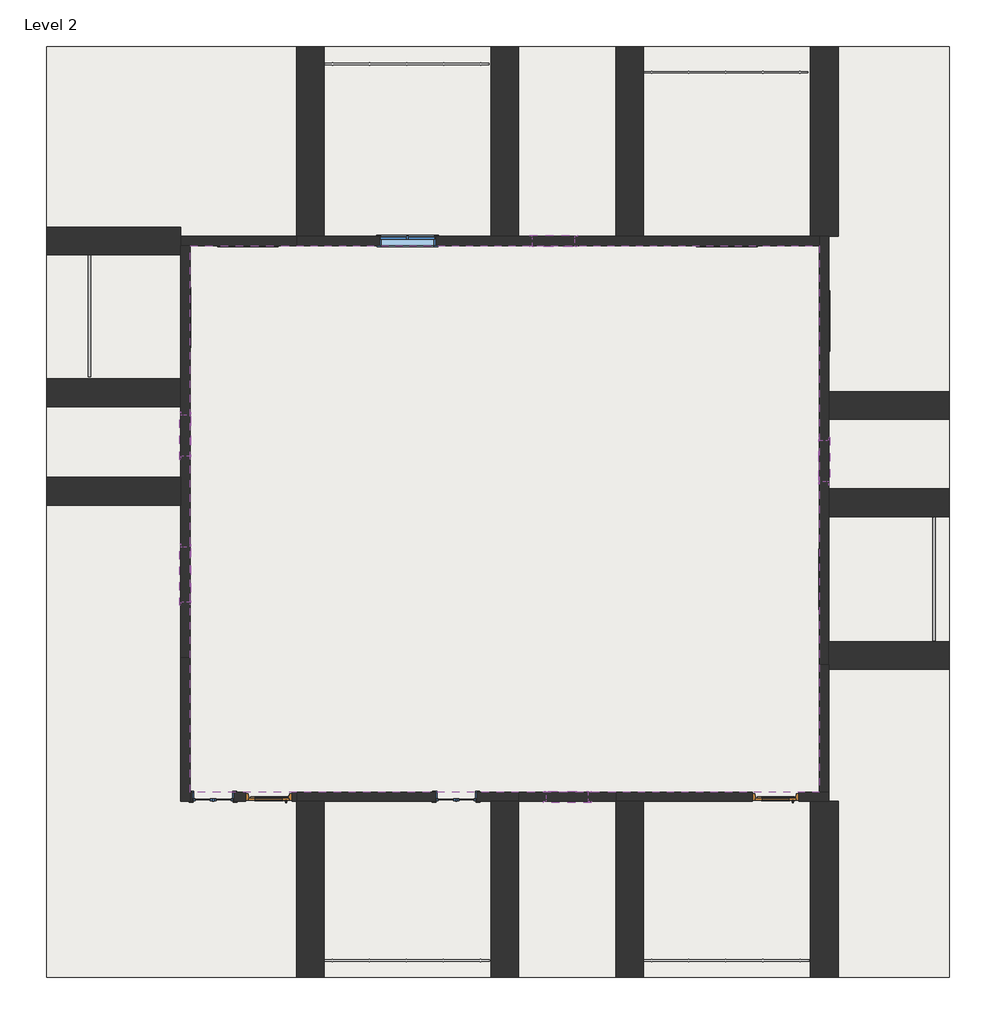
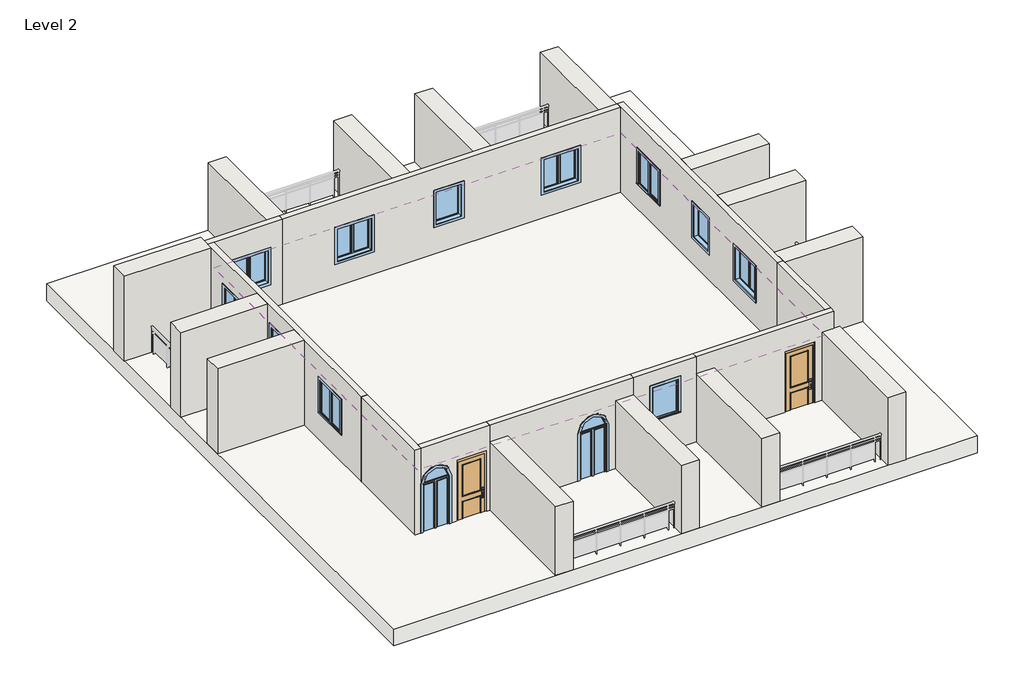
# One storey, part 1 of 2: 24 walls, 13 windows, 2 doors, 1 covering, 1 slab.
"""IFC4 building model written with IfcOpenShell, lengths in millimetres."""

from ifc_helpers import new_model, si_unit, point, frame, frame_2d, origin, place, context, project, spatial, polyline, circle_curve, trimmed, segment, composite_curve, outline, extrude, faceted_brep, transform, mapped, element, save
from ifc_brep_helpers import plane_surface, revolved_surface, advanced_brep
from components import door_b6c2ee01, window_4e95f2a8, window_0862ab64, window_3a1167bf, window_8a4441b2

model = new_model("IFC4")

# Units and contexts
model_context = context("Model", 3, world=origin())
ifc_project = project(units=[si_unit("LENGTHUNIT", "METRE", prefix="MILLI")], contexts=[model_context])

# Site, building, storey
site = spatial("IfcSite", under=ifc_project)
building = spatial("IfcBuilding", under=site)
storey = spatial("IfcBuildingStorey", under=building, Name="Level 2", Elevation=3048.0)

# Covering
placement = place(None, origin())
element("IfcCovering", 1, ObjectType="2' x 4' ACT System", at=placement, inside=storey, context=model_context, shape_type="SweptSolid", body=[
    extrude(outline(polyline([(-12179.4937431, 6319.013611), (-9842.6937431, 6319.013611), (1638.1062569, 6319.013611), (1638.1062569, -2875.786389), (1638.1062569, -5669.786389), (-2832.2937431, -5669.786389), (-4965.8937431, -5669.786389), (-9842.6937431, -5669.786389), (-12179.4937431, -5669.786389), (-12179.4937431, -2723.386389), (-12179.4937431, 6319.013611)])), frame((0.0, 0.0, 5486.4), z_axis=(0.0, 0.0, 1.0), x_axis=(1.0, 0.0, 0.0)), (0.0, 0.0, 1.0), 57.15),
])

# Doors
door_shape = door_b6c2ee01(model_context)
element("IfcDoor", 2, ObjectType="Door-Exterior-Single-Two_Lite : 36\" x 94\"", at=placement, inside=storey, context=model_context, shape_type="MappedRepresentation", body=[
    mapped(door_shape, transform((-10452.2937431, -5765.036389, 3048.0), x_axis=(-1.0, 0.0, 0.0), y_axis=(0.0, -1.0, 0.0), z_axis=(0.0, 0.0, 1.0))),
])
element("IfcDoor", 3, ObjectType="Door-Exterior-Single-Two_Lite : 36\" x 94\"", at=placement, inside=storey, context=model_context, shape_type="MappedRepresentation", body=[
    mapped(door_shape, transform((672.9062569, -5765.036389, 3048.0), x_axis=(-1.0, 0.0, 0.0), y_axis=(0.0, -1.0, 0.0), z_axis=(0.0, 0.0, 1.0))),
])

# Slab
element("IfcSlab", 4, ObjectType="Generic - 2' 4", at=placement, inside=storey, context=model_context, shape_type="SweptSolid", body=[
    extrude(outline(polyline([(4482.9062569, 10687.813611), (4482.9062569, -9733.786389), (-15329.0937431, -9733.786389), (-15329.0937431, 10687.813611), (4482.9062569, 10687.813611)])), frame((0.0, 0.0, 2743.2), z_axis=(0.0, 0.0, 1.0), x_axis=(1.0, 0.0, 0.0)), (0.0, 0.0, 1.0), 609.6),
])

# Walls
element("IfcWall", 5, ObjectType="Generic - 8\"", at=placement, inside=storey, context=model_context, shape_type="Brep", body=[
    faceted_brep([(-12382.6937431, 6319.013611, 3352.8), (-12179.4937431, 6319.013611, 3352.8), (-9842.6937431, 6319.013611, 3352.8), (-9842.6937431, 6319.013611, 6400.8), (-12179.4937431, 6319.013611, 6400.8), (-12382.6937431, 6319.013611, 6400.8), (-10299.8937431, 6319.013611, 5486.4), (-10299.8937431, 6319.013611, 4267.2), (-11519.0937431, 6319.013611, 4267.2), (-11519.0937431, 6319.013611, 5486.4), (-12382.6937431, 6522.213611, 3352.8), (-12382.6937431, 6522.213611, 6400.8), (-9842.6937431, 6522.213611, 6400.8), (-9842.6937431, 6522.213611, 3352.8), (-10299.8937431, 6522.213611, 5486.4), (-11519.0937431, 6522.213611, 5486.4), (-11519.0937431, 6522.213611, 4267.2), (-10299.8937431, 6522.213611, 4267.2)], [[[0, 1, 2, 3, 4, 5], [6, 7, 8, 9]], [[10, 11, 12, 13], [14, 15, 16, 17]], [[2, 1, 0, 10, 13]], [[3, 2, 13, 12]], [[5, 4, 3, 12, 11]], [[0, 5, 11, 10]], [[7, 6, 14, 17]], [[8, 7, 17, 16]], [[9, 8, 16, 15]], [[6, 9, 15, 14]]]),
])
element("IfcWall", 6, ObjectType="Generic - 8\"", at=placement, inside=storey, context=model_context, shape_type="Brep", body=[
    faceted_brep([(-12179.4937431, -5872.986389, 3352.8), (-12179.4937431, -5669.786389, 3352.8), (-12179.4937431, -2723.386389, 3352.8), (-12179.4937431, -2723.386389, 6400.8), (-12179.4937431, -5669.786389, 6400.8), (-12179.4937431, -5872.986389, 6400.8), (-12382.6937431, -5872.986389, 3352.8), (-12382.6937431, -5872.986389, 6400.8), (-12382.6937431, -2723.386389, 6400.8), (-12382.6937431, -2723.386389, 3352.8)], [[[0, 1, 2, 3, 4, 5]], [[6, 7, 8, 9]], [[2, 1, 0, 6, 9]], [[3, 2, 9, 8]], [[5, 4, 3, 8, 7]], [[0, 5, 7, 6]]]),
])
element("IfcWall", 7, ObjectType="Generic - 8\"", at=placement, inside=storey, context=model_context, shape_type="Brep", body=[
    faceted_brep([(-2832.2937431, -5669.786389, 3352.8), (-2832.2937431, -5669.786389, 6400.8), (1638.1062569, -5669.786389, 6400.8), (1841.3062569, -5669.786389, 6400.8), (1841.3062569, -5669.786389, 3352.8), (1638.1062569, -5669.786389, 3352.8), (1180.9062569, -5669.786389, 3352.8), (1180.9062569, -5669.786389, 5537.2), (164.9062569, -5669.786389, 5537.2), (164.9062569, -5669.786389, 3352.8), (-2832.2937431, -5872.986389, 6400.8), (-2832.2937431, -5872.986389, 5798.8571637), (-2832.2937431, -5872.986389, 3352.8), (-2222.6937431, -5872.986389, 3352.8), (164.9062569, -5872.986389, 3352.8), (164.9062569, -5872.986389, 5537.2), (1180.9062569, -5872.986389, 5537.2), (1180.9062569, -5872.986389, 3352.8), (1434.9062569, -5872.986389, 3352.8), (1841.3062569, -5872.986389, 3352.8), (1841.3062569, -5872.986389, 6400.8)], [[[0, 1, 2, 3, 4, 5, 6, 7, 8, 9]], [[10, 11, 12, 13, 14, 15, 16, 17, 18, 19, 20]], [[4, 19, 18, 17, 6, 5]], [[12, 0, 9, 14, 13]], [[1, 0, 12, 11, 10]], [[3, 2, 1, 10, 20]], [[3, 20, 19, 4]], [[8, 15, 14, 9]], [[15, 8, 7, 16]], [[16, 7, 6, 17]]]),
])
element("IfcWall", 8, ObjectType="Generic - 8\"", at=placement, inside=storey, context=model_context, shape_type="Brep", body=[
    faceted_brep([(1638.1062569, 6522.213611, 6400.8), (1638.1062569, 6522.213611, 3352.8), (1638.1062569, 6319.013611, 3352.8), (1638.1062569, -2875.786389, 3352.8), (1638.1062569, -2875.786389, 6400.8), (1638.1062569, 6319.013611, 6400.8), (1638.1062569, 1137.413611, 5557.6747769), (1638.1062569, 1137.413611, 4338.4747769), (1638.1062569, 2051.813611, 4338.4747769), (1638.1062569, 2051.813611, 5557.6747769), (1638.1062569, -1605.786389, 5497.5712595), (1638.1062569, -1605.786389, 4278.3712595), (1638.1062569, -386.586389, 4278.3712595), (1638.1062569, -386.586389, 5497.5712595), (1638.1062569, 4058.413611, 5497.5712595), (1638.1062569, 4058.413611, 4278.3712595), (1638.1062569, 5277.613611, 4278.3712595), (1638.1062569, 5277.613611, 5497.5712595), (1841.3062569, 6522.213611, 3352.8), (1841.3062569, 6522.213611, 6400.8), (1841.3062569, 3118.613611, 6400.8), (1841.3062569, 2509.013611, 6400.8), (1841.3062569, 985.013611, 6400.8), (1841.3062569, 375.413611, 6400.8), (1841.3062569, -2367.786389, 6400.8), (1841.3062569, -2875.786389, 6400.8), (1841.3062569, -2875.786389, 3352.8), (1841.3062569, -2367.786389, 3352.8), (1841.3062569, 375.413611, 3352.8), (1841.3062569, 985.013611, 3352.8), (1841.3062569, 2509.013611, 3352.8), (1841.3062569, 3118.613611, 3352.8), (1841.3062569, 1137.413611, 5557.6747769), (1841.3062569, 2051.813611, 5557.6747769), (1841.3062569, 2051.813611, 4338.4747769), (1841.3062569, 1137.413611, 4338.4747769), (1841.3062569, -1605.786389, 5497.5712595), (1841.3062569, -386.586389, 5497.5712595), (1841.3062569, -386.586389, 4278.3712595), (1841.3062569, -1605.786389, 4278.3712595), (1841.3062569, 4058.413611, 5497.5712595), (1841.3062569, 5277.613611, 5497.5712595), (1841.3062569, 5277.613611, 4278.3712595), (1841.3062569, 4058.413611, 4278.3712595)], [[[0, 1, 2, 3, 4, 5], [6, 7, 8, 9], [10, 11, 12, 13], [14, 15, 16, 17]], [[18, 19, 20, 21, 22, 23, 24, 25, 26, 27, 28, 29, 30, 31], [32, 33, 34, 35], [36, 37, 38, 39], [40, 41, 42, 43]], [[3, 2, 1, 18, 31, 30, 29, 28, 27, 26]], [[4, 3, 26, 25]], [[0, 5, 4, 25, 24, 23, 22, 21, 20, 19]], [[0, 19, 18, 1]], [[7, 6, 32, 35]], [[8, 7, 35, 34]], [[9, 8, 34, 33]], [[6, 9, 33, 32]], [[11, 10, 36, 39]], [[12, 11, 39, 38]], [[13, 12, 38, 37]], [[10, 13, 37, 36]], [[15, 14, 40, 43]], [[16, 15, 43, 42]], [[17, 16, 42, 41]], [[14, 17, 41, 40]]]),
])
element("IfcWall", 9, ObjectType="Generic - 8\"", at=placement, inside=storey, context=model_context, shape_type="Brep", body=[
    faceted_brep([(-12179.4937431, -2723.386389, 3352.8), (-12179.4937431, 6319.013611, 3352.8), (-12179.4937431, 6319.013611, 6400.8), (-12179.4937431, -2723.386389, 6400.8), (-12179.4937431, 2610.613611, 5723.7149116), (-12179.4937431, 2610.613611, 4504.5149116), (-12179.4937431, 1696.213611, 4504.5149116), (-12179.4937431, 1696.213611, 5723.7149116), (-12179.4937431, -284.986389, 5546.8059909), (-12179.4937431, -284.986389, 4327.6059909), (-12179.4937431, -1504.186389, 4327.6059909), (-12179.4937431, -1504.186389, 5546.8059909), (-12179.4937431, 5353.813611, 5473.1335827), (-12179.4937431, 5353.813611, 4253.9335827), (-12179.4937431, 4134.613611, 4253.9335827), (-12179.4937431, 4134.613611, 5473.1335827), (-12382.6937431, -2723.386389, 3352.8), (-12382.6937431, -2723.386389, 6400.8), (-12382.6937431, 629.413611, 6400.8), (-12382.6937431, 1239.013611, 6400.8), (-12382.6937431, 2788.413611, 6400.8), (-12382.6937431, 3398.013611, 6400.8), (-12382.6937431, 6115.813611, 6400.8), (-12382.6937431, 6319.013611, 6400.8), (-12382.6937431, 6319.013611, 3352.8), (-12382.6937431, 6115.813611, 3352.8), (-12382.6937431, 3398.013611, 3352.8), (-12382.6937431, 2788.413611, 3352.8), (-12382.6937431, 1239.013611, 3352.8), (-12382.6937431, 629.413611, 3352.8), (-12382.6937431, 2610.613611, 5723.7149116), (-12382.6937431, 1696.213611, 5723.7149116), (-12382.6937431, 1696.213611, 4504.5149116), (-12382.6937431, 2610.613611, 4504.5149116), (-12382.6937431, -284.986389, 5546.8059909), (-12382.6937431, -1504.186389, 5546.8059909), (-12382.6937431, -1504.186389, 4327.6059909), (-12382.6937431, -284.986389, 4327.6059909), (-12382.6937431, 5353.813611, 5473.1335827), (-12382.6937431, 4134.613611, 5473.1335827), (-12382.6937431, 4134.613611, 4253.9335827), (-12382.6937431, 5353.813611, 4253.9335827)], [[[0, 1, 2, 3], [4, 5, 6, 7], [8, 9, 10, 11], [12, 13, 14, 15]], [[16, 17, 18, 19, 20, 21, 22, 23, 24, 25, 26, 27, 28, 29], [30, 31, 32, 33], [34, 35, 36, 37], [38, 39, 40, 41]], [[1, 0, 16, 29, 28, 27, 26, 25, 24]], [[3, 2, 23, 22, 21, 20, 19, 18, 17]], [[0, 3, 17, 16]], [[2, 1, 24, 23]], [[5, 4, 30, 33]], [[6, 5, 33, 32]], [[7, 6, 32, 31]], [[4, 7, 31, 30]], [[9, 8, 34, 37]], [[10, 9, 37, 36]], [[11, 10, 36, 35]], [[8, 11, 35, 34]], [[13, 12, 38, 41]], [[14, 13, 41, 40]], [[15, 14, 40, 39]], [[12, 15, 39, 38]]]),
])
element("IfcWall", 10, ObjectType="Generic - 8\"", at=placement, inside=storey, context=model_context, shape_type="SweptSolid", body=[
    extrude(outline(composite_curve([segment(polyline([(6400.8, -9842.6937431), (6400.8, -12179.4937431), (3352.8, -12179.4937431), (3352.8, -12128.6937431), (5091.597687, -12128.6937431)]), True, "CONTINUOUS"), segment(trimmed(circle_curve(frame_2d((5091.597687, -11671.4937431)), 457.2), [point((5091.597687, -12128.6937431))], [point((5091.597687, -11214.2937431))], True, "CARTESIAN"), True, "CONTINUOUS"), segment(polyline([(5091.597687, -11214.2937431), (3352.8, -11214.2937431), (3352.8, -10960.2937431), (5537.2, -10960.2937431), (5537.2, -9944.2937431), (3352.8, -9944.2937431), (3352.8, -9842.6937431), (6400.8, -9842.6937431)]), True, "CONTINUOUS")], self_intersect=False)), frame((0.0, -5872.986389, 0.0), z_axis=(0.0, 1.0, 0.0), x_axis=(0.0, 0.0, 1.0)), (0.0, 0.0, 1.0), 203.2),
])
element("IfcWall", 11, ObjectType="Generic - 8\"", at=placement, inside=storey, context=model_context, shape_type="SweptSolid", body=[
    extrude(outline(polyline([(1638.1062569, -5669.786389), (1638.1062569, -2875.786389), (1841.3062569, -2875.786389), (1841.3062569, -5669.786389), (1638.1062569, -5669.786389)])), frame((0.0, 0.0, 3352.8), z_axis=(0.0, 0.0, 1.0), x_axis=(1.0, 0.0, 0.0)), (0.0, 0.0, 1.0), 3048.0),
])
element("IfcWall", 12, ObjectType="Generic - 8\"", at=placement, inside=storey, context=model_context, shape_type="Brep", body=[
    faceted_brep([(-9842.6937431, 6319.013611, 3352.8), (1638.1062569, 6319.013611, 3352.8), (1638.1062569, 6319.013611, 6400.8), (-9842.6937431, 6319.013611, 6400.8), (-3746.6937431, 6319.013611, 5584.3983257), (-3746.6937431, 6319.013611, 4365.1983257), (-4661.0937431, 6319.013611, 4365.1983257), (-4661.0937431, 6319.013611, 5584.3983257), (-6794.6937431, 6319.013611, 5433.182989), (-6794.6937431, 6319.013611, 4213.982989), (-8013.8937431, 6319.013611, 4213.982989), (-8013.8937431, 6319.013611, 5433.182989), (215.7062569, 6319.013611, 5470.4159819), (215.7062569, 6319.013611, 4251.2159819), (-1003.4937431, 6319.013611, 4251.2159819), (-1003.4937431, 6319.013611, 5470.4159819), (-9842.6937431, 6522.213611, 3352.8), (-9842.6937431, 6522.213611, 5791.2), (-9842.6937431, 6522.213611, 6400.8), (1638.1062569, 6522.213611, 6400.8), (1638.1062569, 6522.213611, 3352.8), (1434.9062569, 6522.213611, 3352.8), (-2222.6937431, 6522.213611, 3352.8), (-2832.2937431, 6522.213611, 3352.8), (-4965.8937431, 6522.213611, 3352.8), (-5575.4937431, 6522.213611, 3352.8), (-9233.0937431, 6522.213611, 3352.8), (-3746.6937431, 6522.213611, 5584.3983257), (-4661.0937431, 6522.213611, 5584.3983257), (-4661.0937431, 6522.213611, 4365.1983257), (-3746.6937431, 6522.213611, 4365.1983257), (-6794.6937431, 6522.213611, 5433.182989), (-8013.8937431, 6522.213611, 5433.182989), (-8013.8937431, 6522.213611, 4213.982989), (-6794.6937431, 6522.213611, 4213.982989), (215.7062569, 6522.213611, 5470.4159819), (-1003.4937431, 6522.213611, 5470.4159819), (-1003.4937431, 6522.213611, 4251.2159819), (215.7062569, 6522.213611, 4251.2159819)], [[[0, 1, 2, 3], [4, 5, 6, 7], [8, 9, 10, 11], [12, 13, 14, 15]], [[16, 17, 18, 19, 20, 21, 22, 23, 24, 25, 26], [27, 28, 29, 30], [31, 32, 33, 34], [35, 36, 37, 38]], [[1, 0, 16, 26, 25, 24, 23, 22, 21, 20]], [[3, 2, 19, 18]], [[0, 3, 18, 17, 16]], [[1, 20, 19, 2]], [[5, 4, 27, 30]], [[6, 5, 30, 29]], [[7, 6, 29, 28]], [[4, 7, 28, 27]], [[9, 8, 31, 34]], [[10, 9, 34, 33]], [[11, 10, 33, 32]], [[8, 11, 32, 31]], [[13, 12, 35, 38]], [[14, 13, 38, 37]], [[15, 14, 37, 36]], [[12, 15, 36, 35]]]),
])
element("IfcWall", 13, ObjectType="Generic - 8\"", at=placement, inside=storey, context=model_context, shape_type="SweptSolid", body=[
    extrude(outline(polyline([(3352.8, -2832.2937431), (6400.8, -2832.2937431), (6400.8, -4965.8937431), (3352.8, -4965.8937431), (3352.8, -2832.2937431)]), holes=[polyline([(5847.074951, -4356.2937431), (5847.074951, -3441.8937431), (4627.874951, -3441.8937431), (4627.874951, -4356.2937431), (5847.074951, -4356.2937431)])]), frame((0.0, -5872.986389, 0.0), z_axis=(0.0, 1.0, 0.0), x_axis=(0.0, 0.0, 1.0)), (0.0, 0.0, 1.0), 203.2),
])
element("IfcWall", 14, ObjectType="Generic - 8\"", at=placement, inside=storey, context=model_context, shape_type="AdvancedBrep", body=[
    advanced_brep(
    [(-9842.6937431, -5669.786389, 3352.8), (-9842.6937431, -5669.786389, 6400.8), (-4965.8937431, -5669.786389, 6400.8), (-4965.8937431, -5669.786389, 3352.8), (-5880.2937431, -5669.786389, 3352.8), (-5880.2937431, -5669.786389, 5048.25), (-6794.6937431, -5669.786389, 5048.25), (-6794.6937431, -5669.786389, 3352.8), (-9842.6937431, -5872.986389, 6400.8), (-9842.6937431, -5872.986389, 5811.7612992), (-9842.6937431, -5872.986389, 3352.8), (-9233.0937431, -5872.986389, 3352.8), (-6794.6937431, -5872.986389, 3352.8), (-6794.6937431, -5872.986389, 5048.25), (-5880.2937431, -5872.986389, 5048.25), (-5880.2937431, -5872.986389, 3352.8), (-5575.4937431, -5872.986389, 3352.8), (-4965.8937431, -5872.986389, 3352.8), (-4965.8937431, -5872.986389, 5791.2), (-4965.8937431, -5872.986389, 6400.8)],
    [
        (0, 1),
        (1, 2),
        (2, 3),
        (3, 4),
        (4, 5),
        (5, 6, circle_curve(frame((-6337.4937431, -5669.786389, 5048.25), z_axis=(0.0, -1.0, 0.0), x_axis=(-1.0, 0.0, 0.0)), 457.2)),
        (6, 7),
        (7, 0),
        (8, 9),
        (9, 10),
        (10, 11),
        (11, 12),
        (12, 13),
        (13, 14, circle_curve(frame((-6337.4937431, -5872.986389, 5048.25), z_axis=(0.0, 1.0, 0.0), x_axis=(-1.0, 0.0, 0.0)), 457.2)),
        (14, 15),
        (15, 16),
        (16, 17),
        (17, 18),
        (18, 19),
        (19, 8),
        (3, 17),
        (15, 4),
        (10, 0),
        (7, 12),
        (8, 1),
        (19, 2),
        (6, 13),
        (14, 5),
    ],
    [
        plane_surface(frame((1423.3958892, -5669.786389, 3352.8), z_axis=(0.0, 1.0, 0.0), x_axis=(-1.0, 0.0, 0.0))),
        plane_surface(frame((1423.3958892, -5872.986389, 3352.8), z_axis=(0.0, -1.0, 0.0), x_axis=(1.0, 0.0, 0.0))),
        plane_surface(frame((-4965.8937431, -5669.786389, 3352.8), z_axis=(0.0, 0.0, -1.0), x_axis=(0.0, -1.0, 0.0))),
        plane_surface(frame((-9842.6937431, -5669.786389, 3352.8), z_axis=(-1.0, 0.0, 0.0), x_axis=(0.0, -1.0, 0.0))),
        plane_surface(frame((-9842.6937431, -5669.786389, 6400.8), z_axis=(0.0, 0.0, 1.0), x_axis=(0.0, -1.0, 0.0))),
        plane_surface(frame((-4965.8937431, -5669.786389, 6400.8), z_axis=(1.0, 0.0, 0.0), x_axis=(0.0, -1.0, 0.0))),
        plane_surface(frame((-6794.6937431, -7193.786389, 5048.25), z_axis=(1.0, 0.0, 0.0), x_axis=(0.0, 1.0, 0.0))),
        plane_surface(frame((-5880.2937431, -7193.786389, 3200.4), z_axis=(-1.0, 0.0, 0.0), x_axis=(0.0, 1.0, 0.0))),
        revolved_surface(polyline([(-6794.6937431, -5872.986389, 5048.25), (-6794.6937431, -5669.786389, 5048.25)]), (-6337.4937431, -4145.786389, 5048.25), (0.0, -1.0, 0.0)),
    ],
    [
        (0, [[1, 2, 3, 4, 5, 6, 7, 8]]),
        (1, [[9, 10, 11, 12, 13, 14, 15, 16, 17, 18, 19, 20]]),
        (2, [[21, -17, -16, 22, -4]]),
        (2, [[23, -8, 24, -12, -11]]),
        (3, [[-1, -23, -10, -9, 25]]),
        (4, [[-2, -25, -20, 26]]),
        (5, [[-3, -26, -19, -18, -21]]),
        (6, [[27, -13, -24, -7]]),
        (7, [[28, -5, -22, -15]]),
        (8, [[-27, -6, -28, -14]]),
    ],
),
])
element("IfcWall", 15, ObjectType="Generic -2' 2", at=placement, inside=storey, context=model_context, shape_type="Brep", body=[
    faceted_brep([(-12382.6937431, 6725.413611, 3352.8), (-15329.0937431, 6725.413611, 3352.8), (-15329.0937431, 6725.413611, 6400.8), (-12382.6937431, 6725.413611, 6400.8), (-12382.6937431, 6115.813611, 3352.8), (-12382.6937431, 6115.813611, 6400.8), (-15329.0937431, 6115.813611, 6400.8), (-15329.0937431, 6115.813611, 3352.8), (-12382.6937431, 6522.213611, 3352.8), (-12382.6937431, 6319.013611, 3352.8), (-12382.6937431, 6319.013611, 6400.8), (-12382.6937431, 6522.213611, 6400.8)], [[[0, 1, 2, 3]], [[4, 5, 6, 7]], [[1, 0, 8, 9, 4, 7]], [[2, 1, 7, 6]], [[3, 2, 6, 5, 10, 11]], [[0, 3, 11, 10, 5, 4, 9, 8]]]),
])
element("IfcWall", 16, ObjectType="Generic -2' 2", at=placement, inside=storey, context=model_context, shape_type="SweptSolid", body=[
    extrude(outline(polyline([(-15329.0937431, 3398.013611), (-12382.6937431, 3398.013611), (-12382.6937431, 2788.413611), (-15329.0937431, 2788.413611), (-15329.0937431, 3398.013611)])), frame((0.0, 0.0, 3352.8), z_axis=(0.0, 0.0, 1.0), x_axis=(1.0, 0.0, 0.0)), (0.0, 0.0, 1.0), 3048.0),
])
element("IfcWall", 17, ObjectType="Generic -2' 2", at=placement, inside=storey, context=model_context, shape_type="SweptSolid", body=[
    extrude(outline(polyline([(-15329.0937431, 1239.013611), (-12382.6937431, 1239.013611), (-12382.6937431, 629.413611), (-15329.0937431, 629.413611), (-15329.0937431, 1239.013611)])), frame((0.0, 0.0, 3352.8), z_axis=(0.0, 0.0, 1.0), x_axis=(1.0, 0.0, 0.0)), (0.0, 0.0, 1.0), 3048.0),
])
element("IfcWall", 18, ObjectType="Generic -2' 2", at=placement, inside=storey, context=model_context, shape_type="Brep", body=[
    faceted_brep([(1841.3062569, -2977.386389, 3352.8), (4482.9062569, -2977.386389, 3352.8), (4482.9062569, -2977.386389, 6400.8), (1841.3062569, -2977.386389, 6400.8), (1841.3062569, -2367.786389, 3352.8), (1841.3062569, -2367.786389, 6400.8), (4482.9062569, -2367.786389, 6400.8), (4482.9062569, -2367.786389, 3352.8), (1841.3062569, -2875.786389, 3352.8), (1841.3062569, -2875.786389, 6400.8)], [[[0, 1, 2, 3]], [[4, 5, 6, 7]], [[1, 0, 8, 4, 7]], [[2, 1, 7, 6]], [[3, 2, 6, 5, 9]], [[0, 3, 9, 5, 4, 8]]]),
])
element("IfcWall", 19, ObjectType="Generic -2' 2", at=placement, inside=storey, context=model_context, shape_type="SweptSolid", body=[
    extrude(outline(polyline([(4482.9062569, 375.413611), (1841.3062569, 375.413611), (1841.3062569, 985.013611), (4482.9062569, 985.013611), (4482.9062569, 375.413611)])), frame((0.0, 0.0, 3352.8), z_axis=(0.0, 0.0, 1.0), x_axis=(1.0, 0.0, 0.0)), (0.0, 0.0, 1.0), 3048.0),
])
element("IfcWall", 20, ObjectType="Generic -2' 2", at=placement, inside=storey, context=model_context, shape_type="SweptSolid", body=[
    extrude(outline(polyline([(4482.9062569, 2509.013611), (1841.3062569, 2509.013611), (1841.3062569, 3118.613611), (4482.9062569, 3118.613611), (4482.9062569, 2509.013611)])), frame((0.0, 0.0, 3352.8), z_axis=(0.0, 0.0, 1.0), x_axis=(1.0, 0.0, 0.0)), (0.0, 0.0, 1.0), 3048.0),
])
element("IfcWall", 21, ObjectType="Generic -2' 3 red", at=placement, inside=storey, context=model_context, shape_type="Brep", body=[
    faceted_brep([(1434.9062569, -5872.986389, 3352.8), (1434.9062569, -9733.786389, 3352.8), (1434.9062569, -9733.786389, 5791.2), (1434.9062569, -5872.986389, 5791.2), (2044.5062569, -5872.986389, 3352.8), (2044.5062569, -5872.986389, 5791.2), (2044.5062569, -9733.786389, 5791.2), (2044.5062569, -9733.786389, 3352.8), (1841.3062569, -5872.986389, 3352.8)], [[[0, 1, 2, 3]], [[4, 5, 6, 7]], [[1, 0, 8, 4, 7]], [[2, 1, 7, 6]], [[3, 2, 6, 5]], [[0, 3, 5, 4, 8]]]),
])
element("IfcWall", 22, ObjectType="Generic -2' 3 red", at=placement, inside=storey, context=model_context, shape_type="SweptSolid", body=[
    extrude(outline(polyline([(-2832.2937431, -9733.786389), (-2832.2937431, -5872.986389), (-2222.6937431, -5872.986389), (-2222.6937431, -9733.786389), (-2832.2937431, -9733.786389)])), frame((0.0, 0.0, 3352.8), z_axis=(0.0, 0.0, 1.0), x_axis=(1.0, 0.0, 0.0)), (0.0, 0.0, 1.0), 2446.0571637),
])
element("IfcWall", 23, ObjectType="Generic -2' 3 red", at=placement, inside=storey, context=model_context, shape_type="SweptSolid", body=[
    extrude(outline(polyline([(-5575.4937431, -9733.786389), (-5575.4937431, -5872.986389), (-4965.8937431, -5872.986389), (-4965.8937431, -9733.786389), (-5575.4937431, -9733.786389)])), frame((0.0, 0.0, 3352.8), z_axis=(0.0, 0.0, 1.0), x_axis=(1.0, 0.0, 0.0)), (0.0, 0.0, 1.0), 2438.4),
])
element("IfcWall", 24, ObjectType="Generic -2' 3 red", at=placement, inside=storey, context=model_context, shape_type="SweptSolid", body=[
    extrude(outline(polyline([(-9842.6937431, -9733.786389), (-9842.6937431, -5872.986389), (-9233.0937431, -5872.986389), (-9233.0937431, -9733.786389), (-9842.6937431, -9733.786389)])), frame((0.0, 0.0, 3352.8), z_axis=(0.0, 0.0, 1.0), x_axis=(1.0, 0.0, 0.0)), (0.0, 0.0, 1.0), 2458.9612992),
])
element("IfcWall", 25, ObjectType="Generic -2' 3 red", at=placement, inside=storey, context=model_context, shape_type="SweptSolid", body=[
    extrude(outline(polyline([(-9233.0937431, 10687.813611), (-9233.0937431, 6522.213611), (-9842.6937431, 6522.213611), (-9842.6937431, 10687.813611), (-9233.0937431, 10687.813611)])), frame((0.0, 0.0, 3352.8), z_axis=(0.0, 0.0, 1.0), x_axis=(1.0, 0.0, 0.0)), (0.0, 0.0, 1.0), 2438.4),
])
element("IfcWall", 26, ObjectType="Generic -2' 3 red", at=placement, inside=storey, context=model_context, shape_type="SweptSolid", body=[
    extrude(outline(polyline([(-4965.8937431, 10687.813611), (-4965.8937431, 6522.213611), (-5575.4937431, 6522.213611), (-5575.4937431, 10687.813611), (-4965.8937431, 10687.813611)])), frame((0.0, 0.0, 3352.8), z_axis=(0.0, 0.0, 1.0), x_axis=(1.0, 0.0, 0.0)), (0.0, 0.0, 1.0), 2443.0998934),
])
element("IfcWall", 27, ObjectType="Generic -2' 3 red", at=placement, inside=storey, context=model_context, shape_type="SweptSolid", body=[
    extrude(outline(polyline([(-2222.6937431, 10687.813611), (-2222.6937431, 6522.213611), (-2832.2937431, 6522.213611), (-2832.2937431, 10687.813611), (-2222.6937431, 10687.813611)])), frame((0.0, 0.0, 3352.8), z_axis=(0.0, 0.0, 1.0), x_axis=(1.0, 0.0, 0.0)), (0.0, 0.0, 1.0), 2443.7584708),
])
element("IfcWall", 28, ObjectType="Generic -2' 3 red", at=placement, inside=storey, context=model_context, shape_type="Brep", body=[
    faceted_brep([(2044.5062569, 6522.213611, 3352.8), (2044.5062569, 10687.813611, 3352.8), (2044.5062569, 10687.813611, 5791.2), (2044.5062569, 6522.213611, 5791.2), (1434.9062569, 6522.213611, 3352.8), (1434.9062569, 6522.213611, 5791.2), (1434.9062569, 10687.813611, 5791.2), (1434.9062569, 10687.813611, 3352.8), (1841.3062569, 6522.213611, 3352.8), (1638.1062569, 6522.213611, 3352.8)], [[[0, 1, 2, 3]], [[4, 5, 6, 7]], [[1, 0, 8, 9, 4, 7]], [[2, 1, 7, 6]], [[3, 2, 6, 5]], [[0, 3, 5, 4, 9, 8]]]),
])

# Windows
window_shape = window_4e95f2a8(model_context)
element("IfcWindow", 29, ObjectType="36\" x 72\"", at=placement, inside=storey, context=model_context, shape_type="MappedRepresentation", body=[
    mapped(window_shape, transform((-11663.491585, -5771.386389, 2938.947687), x_axis=(-1.0, 0.0, 0.0), y_axis=(0.0, -1.0, 0.0), z_axis=(0.0, 0.0, 1.0))),
])
element("IfcWindow", 30, ObjectType="36\" x 72\"", at=placement, inside=storey, context=model_context, shape_type="MappedRepresentation", body=[
    mapped(window_shape, transform((-6329.491585, -5771.386389, 2895.6), x_axis=(-1.0, 0.0, 0.0), y_axis=(0.0, -1.0, 0.0), z_axis=(0.0, 0.0, 1.0))),
])
window_2_shape = window_0862ab64(model_context)
element("IfcWindow", 31, ObjectType="Casement Dbl with Trim.0001 : 48\" x 48\"", at=placement, inside=storey, context=model_context, shape_type="MappedRepresentation", body=[
    mapped(window_2_shape, transform((-12262.0437431, -894.586389, 3413.2059909), x_axis=(0.0, 1.0, 0.0), y_axis=(-1.0, 0.0, 0.0), z_axis=(0.0, 0.0, 1.0))),
])
element("IfcWindow", 32, ObjectType="Casement Dbl with Trim.0001 : 48\" x 48\"", at=placement, inside=storey, context=model_context, shape_type="MappedRepresentation", body=[
    mapped(window_2_shape, transform((-12262.0437431, 4744.213611, 3339.5335827), x_axis=(0.0, 1.0, 0.0), y_axis=(-1.0, 0.0, 0.0), z_axis=(0.0, 0.0, 1.0))),
])
element("IfcWindow", 33, ObjectType="Casement Dbl with Trim.0001 : 48\" x 48\"", at=placement, inside=storey, context=model_context, shape_type="MappedRepresentation", body=[
    mapped(window_2_shape, transform((-7404.2937431, 6401.563611, 3299.582989), x_axis=(1.0, 0.0, 0.0), y_axis=(0.0, 1.0, 0.0), z_axis=(0.0, 0.0, 1.0))),
])
element("IfcWindow", 34, ObjectType="Casement Dbl with Trim.0001 : 48\" x 48\"", at=placement, inside=storey, context=model_context, shape_type="MappedRepresentation", body=[
    mapped(window_2_shape, transform((-393.8937431, 6401.563611, 3336.8159819), x_axis=(1.0, 0.0, 0.0), y_axis=(0.0, 1.0, 0.0), z_axis=(0.0, 0.0, 1.0))),
])
element("IfcWindow", 35, ObjectType="Casement Dbl with Trim.0001 : 48\" x 48\"", at=placement, inside=storey, context=model_context, shape_type="MappedRepresentation", body=[
    mapped(window_2_shape, transform((1720.6562569, -996.186389, 3363.9712595), x_axis=(0.0, -1.0, 0.0), y_axis=(1.0, 0.0, 0.0), z_axis=(0.0, 0.0, 1.0))),
])
element("IfcWindow", 36, ObjectType="Casement Dbl with Trim.0001 : 48\" x 48\"", at=placement, inside=storey, context=model_context, shape_type="MappedRepresentation", body=[
    mapped(window_2_shape, transform((-10909.4937431, 6401.563611, 3352.8), x_axis=(1.0, 0.0, 0.0), y_axis=(0.0, 1.0, 0.0), z_axis=(0.0, 0.0, 1.0))),
])
window_3_shape = window_3a1167bf(model_context)
element("IfcWindow", 37, ObjectType="Casement Dbl with Trim.0001 : 48\" x 48\"", at=placement, inside=storey, context=model_context, shape_type="MappedRepresentation", body=[
    mapped(window_3_shape, transform((1758.7562569, 4668.013611, 3363.9712595), x_axis=(0.0, -1.0, 0.0), y_axis=(1.0, 0.0, 0.0), z_axis=(0.0, 0.0, 1.0))),
])
window_4_shape = window_8a4441b2(model_context)
element("IfcWindow", 38, ObjectType="Casement with Trim : 36\" x 48\"", at=placement, inside=storey, context=model_context, shape_type="MappedRepresentation", body=[
    mapped(window_4_shape, transform((-3899.0937431, -5771.386389, 3713.474951), x_axis=(-1.0, 0.0, 0.0), y_axis=(0.0, -1.0, 0.0), z_axis=(0.0, 0.0, 1.0))),
])
element("IfcWindow", 39, ObjectType="Casement with Trim : 36\" x 48\"", at=placement, inside=storey, context=model_context, shape_type="MappedRepresentation", body=[
    mapped(window_4_shape, transform((-12281.0937431, 2153.413611, 3590.1149116), x_axis=(0.0, 1.0, 0.0), y_axis=(-1.0, 0.0, 0.0), z_axis=(0.0, 0.0, 1.0))),
])
element("IfcWindow", 40, ObjectType="Casement with Trim : 36\" x 48\"", at=placement, inside=storey, context=model_context, shape_type="MappedRepresentation", body=[
    mapped(window_4_shape, transform((-4203.8937431, 6420.613611, 3450.7983257), x_axis=(1.0, 0.0, 0.0), y_axis=(0.0, 1.0, 0.0), z_axis=(0.0, 0.0, 1.0))),
])
element("IfcWindow", 41, ObjectType="Casement with Trim : 36\" x 48\"", at=placement, inside=storey, context=model_context, shape_type="MappedRepresentation", body=[
    mapped(window_4_shape, transform((1739.7062569, 1594.613611, 3424.0747769), x_axis=(0.0, -1.0, 0.0), y_axis=(1.0, 0.0, 0.0), z_axis=(0.0, 0.0, 1.0))),
])

save(model, "model.ifc")

# Revit data of these elements
# Type "2' x 4' ACT System"
#   Assembly Code = "C3030210"
#   built-in parameter 1002203 = 1 (stored number, unit not read)
#   built-in parameter 1002202 = 1 (stored number, unit not read)
#   Layers, outside or top first: 0' - 1 5/8" "Default" (function 1); 0' - 0 5/8" "Acoustic Ceiling Tile 24 x 48" (function 5)
# Type "Door-Exterior-Single-Two_Lite : 36\" x 94\""
#   Type Mark = "9"
#   Assembly Code = "B2030100"
#   Analytic Construction = "Metal frame, double glass door"
#   Top Rail = 0' - 6"
#   Threshold Offset [instance default] = 0' - 0 1/2"
#   Threshold Length [instance default] = 3' - 4"
#   Thickness = 0' - 1 3/4"
#   Thermal Resistance (R) = 1.3794 (h·ft²·°F)/BTU
#   Swing Angle [instance default] = 90.00°
#   Strike Height = 3' - 4"
#   Stiles = 0' - 6"
#   Rough Width [instance default] = 3' - 4"
#   Rough Height [instance default] = 8' - 2"
#   MFOpeningHeight [instance default] = 0' - 4"
#   MFOpeningWidth [instance default] = 0' - 4"
#   Lock Rail = 0' - 7 1/2"
#   Heat Transfer Coefficient (U) = 0.7250 BTU/(h·ft²·°F)
#   Glass Thickness = 0' - 0 3/4"
#   Inset Calculate [instance default] = 0' - 4"
#   Masonry Inset [instance default] = 0' - 1"
#   Height = 7' - 10"
#   Width = 3' - 0"
#   Masonry Frame Depth = 0' - 5 3/4"
#   Bottom Rail = 0' - 10"
#   Masonry Frame [instance default] = yes
#   Function = 1
#   Threshold [instance default] = yes
#   Dry Wall Frame [instance default] = no
#   Threshold Material = none
#   Panic Bar Material = Metal - Stainless Steel
#   Panel Material = Metal - Painted - Grey
#   Glass Stop Material = Metal - Painted - Grey
#   Exterior Pull Material = Metal - Stainless Steel
#   Frame Material = Metal - Painted - Grey
#   Visual Light Transmittance = 0
#   Solar Heat Gain Coefficient = 0
#   Wall Closure = (empty or 0)
# Type "Generic - 2' 4"
#   Assembly Code = "B1010"
#   Function = 0
#   Layers, outside or top first: 2' - 0" "Metal - Paint Finish - Grey" (function 1)
# Type "Generic - 8\""
#   Assembly Code = "B2010"
#   Layers, outside or top first: 0' - 8" no material (function 1)
# Type "Generic -2' 2"
#   Assembly Code = "B2010"
#   Layers, outside or top first: 2' - 0" "Damp-proofing" (function 1)
# Type "Generic -2' 3 red"
#   Assembly Code = "B2010"
#   Layers, outside or top first: 2' - 0" "Damp-proofing" (function 1)
# Type "36\" x 72\""
#   Type Mark = "10"
#   Construction Type Id = "SGL"
#   Assembly Code = "B2020100"
#   Analytic Construction = "Large single-glazed windows"
#   Visual Light Transmittance = 0.9
#   Solar Heat Gain Coefficient = 0.86
#   Heat Transfer Coefficient (U) = 0.979472 BTU/(h·ft²·°F)
#   Height = 6' - 0"
#   Default Sill Height = 1' - 0"
#   Trim Projection - Ext. = 0' - 0 1/2"
#   Trim Projection - Int. = 0' - 0 3/4"
#   Trim Width - Exterior = 0' - 3 1/2"
#   Trim Width - Interior = 0' - 3 1/2"
#   Width = 3' - 0"
#   Window Inset = 0' - 0 3/4"
#   Define Thermal Properties by = 1
#   Glass Pane Material = Glass
#   Sash Material = Sash
#   Trim Exterior Material = Trim
#   Trim Interior Material = Trim
#   Wall Closure = (empty or 0)
# Type "Casement Dbl with Trim.0001 : 48\" x 48\""
#   Type Mark = "23"
#   Construction Type Id = "GSP4R"
#   Assembly Code = "B2020100"
#   Analytic Construction = "1/8 in Pilkington single glazing"
#   Visual Light Transmittance = 0.9
#   Solar Heat Gain Coefficient = 0.78
#   Heat Transfer Coefficient (U) = 0.6496 BTU/(h·ft²·°F)
#   Height = 4' - 0"
#   Default Sill Height = 3' - 0"
#   Trim Projection - Ext. = 0' - 0 1/2"
#   Trim Projection - Int. = 0' - 0 3/4"
#   Trim Width - Exterior = 0' - 3 1/2"
#   Trim Width - Interior = 0' - 3 1/2"
#   Width = 4' - 0"
#   Window Inset = 0' - 0 3/4"
#   Define Thermal Properties by = 1
#   Glass Pane Material = Glass
#   Sash Material = Sash
#   Trim Exterior Material = Trim
#   Trim Interior Material = Trim
#   Wall Closure = (empty or 0)
# Type "Casement with Trim : 36\" x 48\""
#   Type Mark = "14"
#   Construction Type Id = "GSP4R"
#   Assembly Code = "B2020100"
#   Analytic Construction = "1/8 in Pilkington single glazing"
#   Visual Light Transmittance = 0.9
#   Solar Heat Gain Coefficient = 0.78
#   Heat Transfer Coefficient (U) = 0.6496 BTU/(h·ft²·°F)
#   Height = 4' - 0"
#   Default Sill Height = 3' - 0"
#   Trim Projection - Ext. = 0' - 0 1/2"
#   Trim Projection - Int. = 0' - 0 3/4"
#   Trim Width - Exterior = 0' - 3 1/2"
#   Trim Width - Interior = 0' - 3 1/2"
#   Width = 3' - 0"
#   Window Inset = 0' - 0 3/4"
#   Define Thermal Properties by = 1
#   Glass Pane Material = Glass
#   Sash Material = Sash
#   Trim Exterior Material = Trim
#   Trim Interior Material = Trim
#   Wall Closure = (empty or 0)
# Element 1 (IfcCovering, "2' x 4' ACT System")
#   Height Offset From Level = 8' - 0"
#   Phase Created = New Construction
#   Materials on its faces: "Acoustic Ceiling Tile 24 x 48", "Default"
# Elements 2, 3 (IfcDoor, "Door-Exterior-Single-Two_Lite : 36\" x 94\"")
#   Threshold Offset = 0' - 0 1/2"
#   Threshold Length = 3' - 4"
#   Swing Angle = 90.00°
#   Rough Width = 3' - 4"
#   Rough Height = 8' - 2"
#   Masonry Inset = 0' - 1"
#   MFOpeningWidth = 0' - 4"
#   MFOpeningHeight = 0' - 4"
#   Inset Calculate = 0' - 4"
#   Threshold = yes
#   Masonry Frame = yes
#   Dry Wall Frame = no
#   Phase Created = New Construction
#   Materials on its faces: "Metal - Painted - Grey", "Metal - Stainless Steel", "Glass"
# Element 4 (IfcSlab, "Generic - 2' 4")
#   Height Offset From Level = 1' - 0"
#   Phase Created = New Construction
#   Materials on its faces: "Gypsum Wall Board", "Metal - Paint Finish - Grey"
# Elements 5, 7, 8, 11, 12, 14 (IfcWall, "Generic - 8\"")
#   built-in parameter 1001111 = 1' - 0"
#   Top Offset = 0' - 0"
#   Base Offset = 1' - 0"
#   Unconnected Height = 10' - 0"
#   wall height = 10' - 0"
#   Phase Created = New Construction
#   Base Constraint = Level 2
#   Materials on its faces: "Default Wall", "Tile, Porcelain, 4in", "Parking Stripe"
# Element 6 (IfcWall, "Generic - 8\"")
#   built-in parameter 1001111 = 1' - 0"
#   Top Offset = 0' - 0"
#   Base Offset = 1' - 0"
#   Unconnected Height = 10' - 0"
#   wall height = 10' - 0"
#   Phase Created = New Construction
#   Base Constraint = Level 2
#   Materials on its faces: "Tile, Porcelain, 4in", "Parking Stripe", "Default Wall"
# Elements 9, 13 (IfcWall, "Generic - 8\"")
#   built-in parameter 1001111 = 1' - 0"
#   Top Offset = 0' - 0"
#   Base Offset = 1' - 0"
#   Unconnected Height = 10' - 0"
#   wall height = 10' - 0"
#   Phase Created = New Construction
#   Base Constraint = Level 2
#   Materials on its faces: "Default Wall", "Tile, Porcelain, 4in"
# Element 10 (IfcWall, "Generic - 8\"")
#   built-in parameter 1001111 = 1' - 0"
#   Top Offset = 0' - 0"
#   Base Offset = 1' - 0"
#   Unconnected Height = 10' - 0"
#   wall height = 10' - 0"
#   Phase Created = New Construction
#   Base Constraint = Level 2
#   Materials on its faces: "Default Wall", "Parking Stripe", "Tile, Porcelain, 4in"
# Elements 15, 16, 17, 18, 19, 20 (IfcWall, "Generic -2' 2")
#   built-in parameter 1001111 = 1' - 0"
#   Top Offset = 0' - 0"
#   Base Offset = 1' - 0"
#   Unconnected Height = 10' - 0"
#   wall height = 10' - 0"
#   Phase Created = New Construction
#   Base Constraint = Level 2
#   Materials on its faces: "Gypsum Wall Board", "Damp-proofing"
# Elements 21, 23, 25, 28 (IfcWall, "Generic -2' 3 red")
#   built-in parameter 1001111 = 1' - 0"
#   Top Offset = 0' - 0"
#   Base Offset = 1' - 0"
#   Unconnected Height = 8' - 0"
#   wall height = 8' - 0"
#   Phase Created = New Construction
#   Base Constraint = Level 2
#   Materials on its faces: "Damp-proofing"
# Element 22 (IfcWall, "Generic -2' 3 red")
#   built-in parameter 1001111 = 1' - 0"
#   Top Offset = 0' - 0"
#   Base Offset = 1' - 0"
#   Unconnected Height = 8' - 0.30146"
#   wall height = 8' - 0.30146"
#   Phase Created = New Construction
#   Base Constraint = Level 2
#   Materials on its faces: "Damp-proofing"
# Element 24 (IfcWall, "Generic -2' 3 red")
#   built-in parameter 1001111 = 1' - 0"
#   Top Offset = 0' - 0"
#   Base Offset = 1' - 0"
#   Unconnected Height = 8' - 0.8095"
#   wall height = 8' - 0.8095"
#   Phase Created = New Construction
#   Base Constraint = Level 2
#   Materials on its faces: "Damp-proofing"
# Element 26 (IfcWall, "Generic -2' 3 red")
#   built-in parameter 1001111 = 1' - 0"
#   Top Offset = 0' - 0"
#   Base Offset = 1' - 0"
#   Unconnected Height = 8' - 0.18504"
#   wall height = 8' - 0.18504"
#   Phase Created = New Construction
#   Base Constraint = Level 2
#   Materials on its faces: "Damp-proofing"
# Element 27 (IfcWall, "Generic -2' 3 red")
#   built-in parameter 1001111 = 1' - 0"
#   Top Offset = 0' - 0"
#   Base Offset = 1' - 0"
#   Unconnected Height = 8' - 0.21096"
#   wall height = 8' - 0.21096"
#   Phase Created = New Construction
#   Base Constraint = Level 2
#   Materials on its faces: "Damp-proofing"
# Element 29 (IfcWindow, "36\" x 72\"")
#   Mark = "1"
#   Phase Created = New Construction
#   Materials on its faces: "Sash", "Trim", "Glass"
# Element 30 (IfcWindow, "36\" x 72\"")
#   Mark = "2"
#   Phase Created = New Construction
#   Materials on its faces: "Sash", "Trim", "Glass"
# Element 31 (IfcWindow, "Casement Dbl with Trim.0001 : 48\" x 48\"")
#   Mark = "7"
#   Phase Created = New Construction
#   Materials on its faces: "Sash", "Trim", "Glass"
# Element 32 (IfcWindow, "Casement Dbl with Trim.0001 : 48\" x 48\"")
#   Mark = "8"
#   Phase Created = New Construction
#   Materials on its faces: "Sash", "Trim", "Glass"
# Element 33 (IfcWindow, "Casement Dbl with Trim.0001 : 48\" x 48\"")
#   Mark = "9"
#   Phase Created = New Construction
#   Materials on its faces: "Sash", "Trim", "Glass"
# Element 34 (IfcWindow, "Casement Dbl with Trim.0001 : 48\" x 48\"")
#   Mark = "10"
#   Phase Created = New Construction
#   Materials on its faces: "Sash", "Trim", "Glass"
# Element 35 (IfcWindow, "Casement Dbl with Trim.0001 : 48\" x 48\"")
#   Mark = "14"
#   Phase Created = New Construction
#   Materials on its faces: "Sash", "Trim", "Glass"
# Element 36 (IfcWindow, "Casement Dbl with Trim.0001 : 48\" x 48\"")
#   Mark = "16"
#   Phase Created = New Construction
#   Materials on its faces: "Sash", "Trim", "Glass"
# Element 37 (IfcWindow, "Casement Dbl with Trim.0001 : 48\" x 48\"")
#   Mark = "15"
#   Phase Created = New Construction
#   Materials on its faces: "Sash", "Trim", "Glass"
# Element 38 (IfcWindow, "Casement with Trim : 36\" x 48\"")
#   Mark = "3"
#   Phase Created = New Construction
#   Materials on its faces: "Sash", "Trim", "Glass"
# Element 39 (IfcWindow, "Casement with Trim : 36\" x 48\"")
#   Mark = "4"
#   Phase Created = New Construction
#   Materials on its faces: "Sash", "Trim", "Glass"
# Element 40 (IfcWindow, "Casement with Trim : 36\" x 48\"")
#   Mark = "5"
#   Phase Created = New Construction
#   Materials on its faces: "Sash", "Trim", "Glass"
# Element 41 (IfcWindow, "Casement with Trim : 36\" x 48\"")
#   Mark = "6"
#   Phase Created = New Construction
#   Materials on its faces: "Sash", "Trim", "Glass"
# Materials
#   "Default": colour RGB 127 127 127, transparency 0
#   "Acoustic Ceiling Tile 24 x 48": class "Generic", colour RGB 229 229 229, transparency 0, Description = "Acoustic Ceiling Tile 24 x 48", Cost = 0
#   "Metal - Stainless Steel": class "Metal", colour RGB 247 247 247, transparency 0
#   "Metal - Painted - Grey": class "Paint", colour RGB 104 104 104, transparency 0
#   "Metal - Paint Finish - Grey": class "Paint", colour RGB 255 255 255, transparency 0, Cost = 0
#   "Damp-proofing": class "Generic", colour RGB 127 127 127, transparency 0, Description = "Damp-proofing", Cost = 0
#   "Glass": class "Glass", colour RGB 0 128 192, transparency 0.75, Description = "Soda Lime Glass", Cost = 0
#   "Sash": class "Wood", colour RGB 224 178 126, transparency 0
#   "Trim": class "Wood", colour RGB 224 178 126, transparency 0
#   "Gypsum Wall Board": class "Generic", colour RGB 127 127 127, transparency 0, Description = "Gypsum Wall Board", Cost = 0
#   "Default Wall": colour RGB 128 128 128, transparency 0
#   "Tile, Porcelain, 4in": class "Generic", colour RGB 89 87 158, transparency 0, Description = "Porcelain tile, 4\", white", Cost = 0
#   "Parking Stripe": class "Paint", colour RGB 250 250 91, transparency 0, Cost = 0
